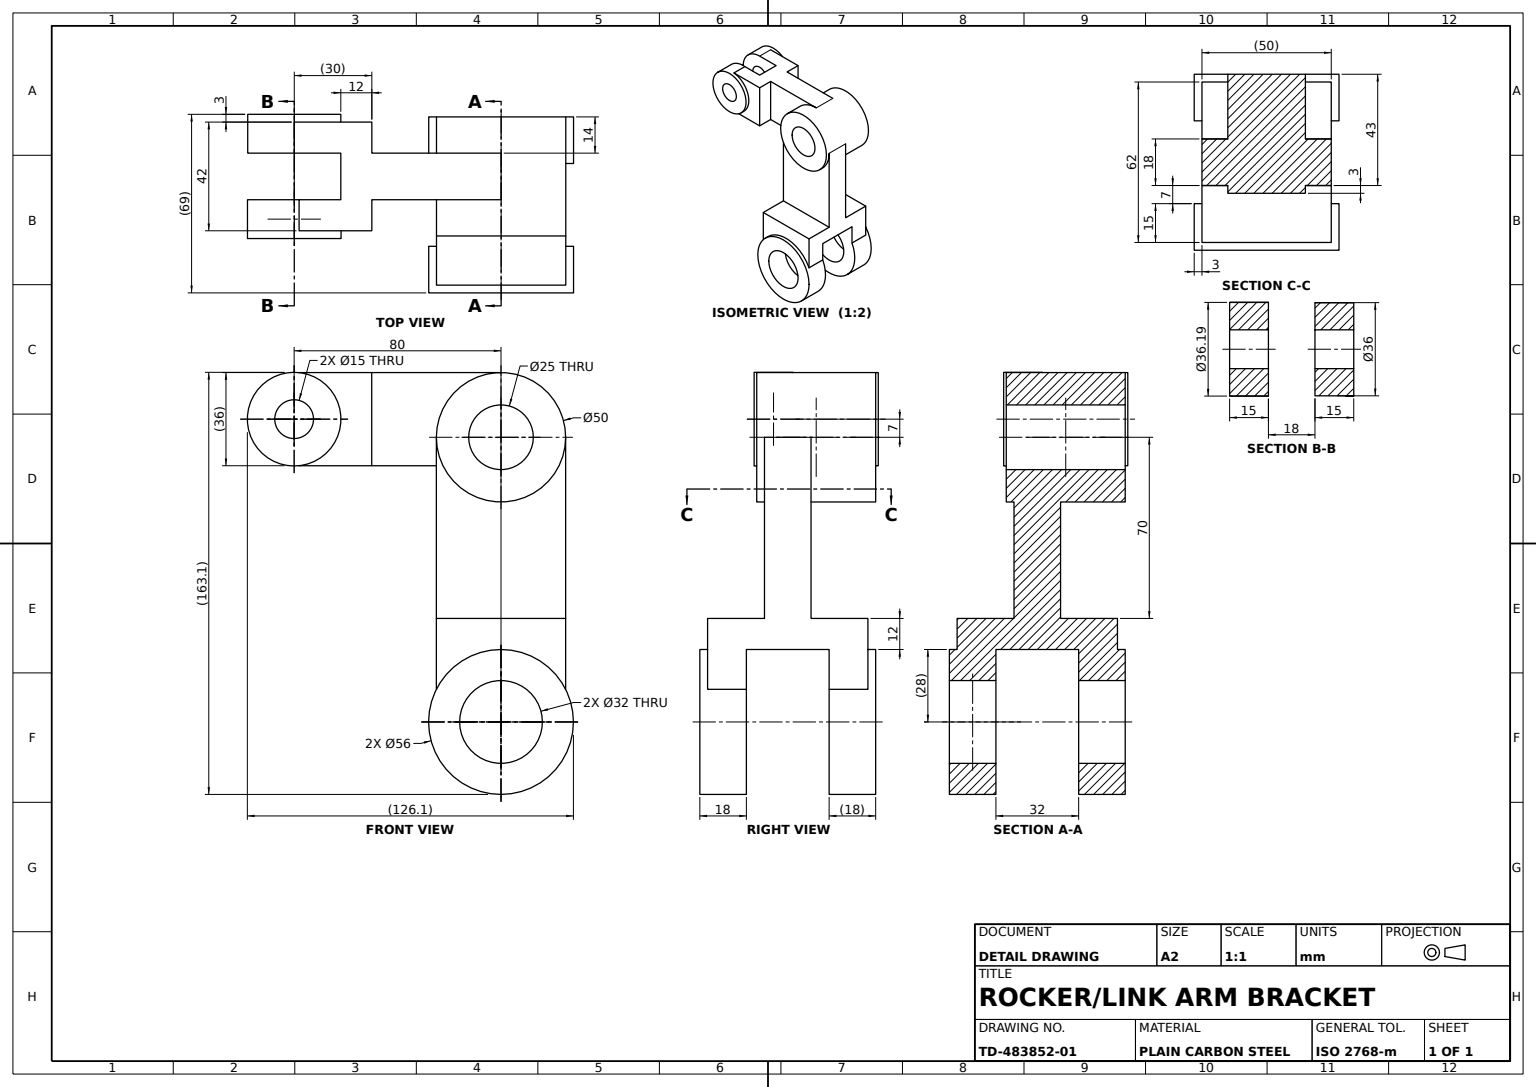
SolidWorks part; units mm, degrees
material "Plain Carbon Steel"
ref_plane "Front Plane" through (0, 0, 0) normal (0, 0, 1) x (1, 0, 0)
ref_plane "Top Plane" through (0, 0, 0) normal (0, 1, 0) x (1, 0, 0)
ref_plane "Right Plane" through (0, 0, 0) normal (1, 0, 0) x (0, 0, -1)
sketch "Base Plate Sketch" plane through (0, 0, 0) normal (0, 1, 0) x (1, 0, 0)
  line L1 (-31, 25) -> (31, 25)
  line L2 (-31, 25) -> (-31, -25)
  line L3 (-31, -25) -> (31, -25)
  line L4 (31, 25) -> (31, -25)
  line L5 (-31, 25) -> (31, -25) construction
  line L6 (-31, -25) -> (31, 25) construction
  point P0 (0, 0)
  dimension "D1" = 62
  dimension "D2" = 50
extrude "Base Plate 62x50x12" add sketch "Base Plate Sketch" along normal blind 12
sketch "Column Sketch" plane through (0, 12, 0) normal (0, 1, 0) x (1, 0, 0)
  line L0 (-9, 25) -> (-9, -25)
  line L1 (31, 25) -> (-31, 25) construction
  line L2 (-31, -25) -> (31, -25) construction
  line L3 (-9, -25) -> (9, -25)
  line L4 (9, -25) -> (9, 25)
  line L5 (9, 25) -> (-9, 25)
  dimension "D1" = 9
  dimension "D2" = 9
extrude "Column 9x9" add sketch "Column Sketch" along normal blind 70
sketch "Upper Hub Sketch" plane through (9, 0, 0) normal (1, 0, 0) x (0, 0, -1)
  line L0 (-25, 82) -> (25, 82) construction
  circle A0 centre (0, 82) radius 25
  circle A1 centre (0, 82) radius 12.5
  dimension "D1" = 50
  dimension "D2" = 25
extrude "Upper Hub" add sketch "Upper Hub Sketch" along normal blind 3 and the other way blind 43
sketch "Lower Ear A Block Sketch" plane through (31, 0, 0) normal (1, 0, 0) x (0, 0, -1)
  line L0 (-25, 0) -> (25, 0)
  line L1 (25, 0) -> (25, -28)
  line L2 (25, -28) -> (-25, -28)
  line L3 (-25, -28) -> (-25, 0)
  dimension "D1" = 28
extrude "Lower Ear A Block" add sketch "Lower Ear A Block Sketch" against normal blind 15
sketch "Lower Ear A Round End Sketch" plane through (31, 0, 0) normal (1, 0, 0) x (0, 0, -1)
  line L0 (-25, -28) -> (25, -28) construction
  circle A0 centre (0, -28) radius 28
  circle A1 centre (0, -28) radius 16
  dimension "D1" = 32
  dimension "D2" = 56
extrude "Lower Ear A Round End" add sketch "Lower Ear A Round End Sketch" against normal blind 15 and the other way blind 3
sketch "Lower Ear A Pin Hole Sketch" plane through (31, 0, 0) normal (1, 0, 0) x (0, 0, -1)
  line L0 (-16, -28) -> (16, -28) construction
  circle A0 centre (0, -28) radius 16
  dimension "D1" = 32
extrude "Lower Ear A Pin Hole" cut sketch "Lower Ear A Pin Hole Sketch" against normal blind 15
sketch "Lower Ear B Block Sketch" plane through (-31, 0, 0) normal (-1, 0, 0) x (0, 0, 1)
  line L0 (-25, 0) -> (-25, -28)
  line L1 (25, 0) -> (25, -28)
  line L2 (25, -28) -> (-25, -28)
  line L3 (-25, 0) -> (25, 0)
  dimension "D1" = 28
extrude "Lower Ear B Block" add sketch "Lower Ear B Block Sketch" against normal blind 15
sketch "Lower Ear B Round End Sketch" plane through (-31, 0, 0) normal (-1, 0, 0) x (0, 0, 1)
  line L0 (-25, -28) -> (25, -28) construction
  circle A0 centre (0, -28) radius 28
  circle A1 centre (0, -28) radius 16
  dimension "D1" = 32
  dimension "D2" = 56
extrude "Lower Ear B Round End" add sketch "Lower Ear B Round End Sketch" against normal blind 15 and the other way blind 3
sketch "Lower Ear B Pin Hole Sketch" plane through (-31, 0, 0) normal (-1, 0, 0) x (0, 0, 1)
  line L0 (-16, -28) -> (16, -28) construction
  circle A0 centre (0, -28) radius 16
  dimension "D1" = 32
extrude "Lower Ear B Pin Hole" cut sketch "Lower Ear B Pin Hole Sketch" against normal blind 15
sketch "Upper Bracket Block Sketch" plane through (0, 0, 25) normal (0, 0, 1) x (1, 0, 0)
  line L0 (-20, 107) -> (-20, 71)
  line L1 (12, 107) -> (-34, 107) construction
  line L2 (-20, 71) -> (-2, 71)
  line L3 (-2, 71) -> (-2, 107)
  line L4 (-2, 107) -> (-20, 107)
  line L5 (12, 57) -> (12, 107) construction
  dimension "D1" = 14
  dimension "D2" = 18
  dimension "D3" = 36
extrude "Upper Bracket Block" add sketch "Upper Bracket Block Sketch" along normal blind 25 and the other way blind 25
sketch "Upper Clevis Arm Sketch" plane through (0, 0, 50) normal (0, 0, 1) x (1, 0, 0)
  line L0 (-20, 107) -> (-20, 71) construction
  line L1 (-2, 107) -> (-20, 107) construction
  line L4 (-32, 107) -> (10, 107)
  line L5 (-32, 107) -> (-32, 71)
  line L6 (-32, 71) -> (10, 71)
  line L7 (10, 107) -> (10, 71)
  line L8 (-32, 107) -> (10, 71) construction
  line L9 (-32, 71) -> (10, 107) construction
  point P6 (-11, 89)
  dimension "D1" = 36
  dimension "D2" = 42
  dimension "D3" = 9
  dimension "D4" = 18
extrude "Upper Clevis Arm" add sketch "Upper Clevis Arm Sketch" along normal blind 30
sketch "Clevis Slot Sketch" plane through (0, 0, 80) normal (0, 0, 1) x (1, 0, 0)
  line L9 (-20, 107) -> (-2, 107)
  line L10 (10, 107) -> (-32, 107) construction
  line L11 (-2, 107) -> (-2, 71)
  line L12 (-32, 71) -> (10, 71) construction
  line L13 (-2, 71) -> (-20, 71)
  line L14 (-20, 71) -> (-20, 107)
  line L15 (10, 71) -> (10, 107) construction
  line L16 (-32, 107) -> (-32, 71) construction
  dimension "D1" = 12
  dimension "D2" = 12
extrude "Clevis Slot 12x12" cut sketch "Clevis Slot Sketch" against normal blind 18
sketch "Upper Ear A Round End Sketch" plane through (10, 0, 0) normal (1, 0, 0) x (0, 0, -1)
  line L0 (-80, 71) -> (-80, 107) construction
  circle A0 centre (-80, 89) radius 18.0962
  circle A1 centre (-80, 89) radius 7.5
  dimension "D1" = 15
  dimension "D2" = 36.1924
extrude "Upper Ear A Round End" add sketch "Upper Ear A Round End Sketch" against normal blind 12 and the other way blind 3
sketch "Upper Ear A Pin Hole Sketch" plane through (10, 0, 0) normal (1, 0, 0) x (0, 0, -1)
  line L0 (-80, 81.5) -> (-80, 96.5) construction
  circle A0 centre (-80, 89) radius 7.5
  dimension "D1" = 15
extrude "Upper Ear A Pin Hole" cut sketch "Upper Ear A Pin Hole Sketch" against normal blind 12
sketch "Upper Ear B Round End Sketch" plane through (-32, 0, 0) normal (-1, 0, 0) x (0, 0, 1)
  line L0 (80, 107) -> (80, 71) construction
  circle A0 centre (80, 89) radius 18
  circle A1 centre (80, 89) radius 7.5
  dimension "D1" = 15
extrude "Upper Ear B Round End" add sketch "Upper Ear B Round End Sketch" against normal blind 12 and the other way blind 3
sketch "Upper Ear B Pin Hole Sketch" plane through (-32, 0, 0) normal (-1, 0, 0) x (0, 0, 1)
  line L0 (80, 96.5) -> (80, 81.5) construction
  circle A0 centre (80, 89) radius 7.5
  dimension "D1" = 15
extrude "Upper Ear B Pin Hole" cut sketch "Upper Ear B Pin Hole Sketch" against normal blind 12
sketch "Hub Bore Sketch" plane through (-34, 0, 0) normal (-1, 0, 0) x (0, 0, 1)
  circle A0 centre (0, 82) radius 12.5
  dimension "D1" = 25
extrude "Hub Bore Through" cut sketch "Hub Bore Sketch" against normal blind 66
